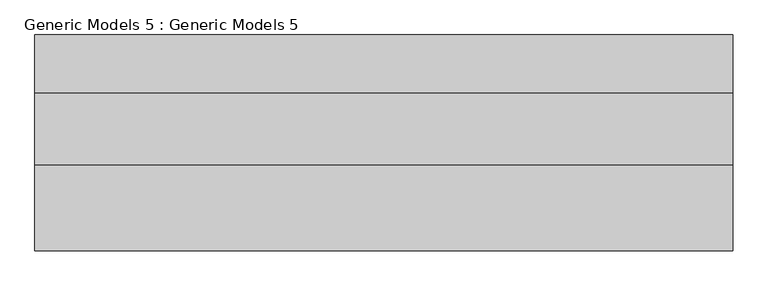
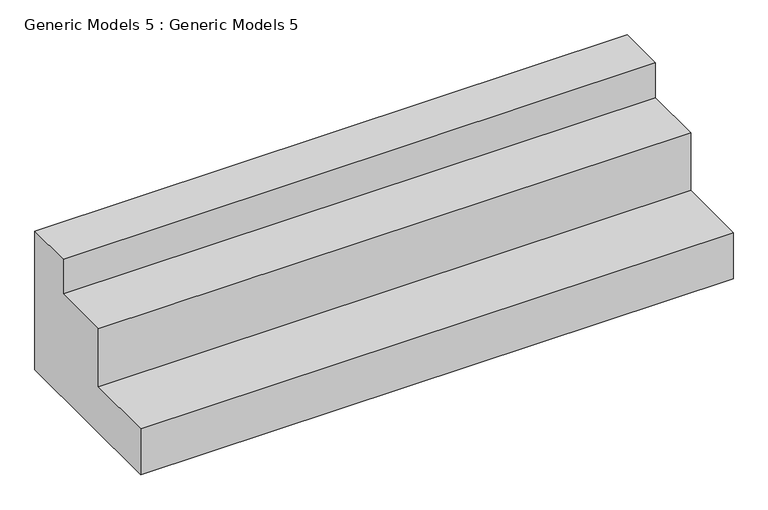
"""IFC4 building model written with IfcOpenShell, lengths in millimetres: proxy geometry, Generic Models 5 : Generic Models 5."""

from ifc_helpers import new_model, si_unit, frame, origin, place, context, project, spatial, polyline, outline, extrude, source, transform, mapped, element, save


def generic_models_5_generic_models_5_28bce95b(model_context):
    return source(origin(), model_context, "Body", "SweptSolid", [
        extrude(outline(polyline([(-4329.7340831, 0.0), (-4710.7340831, 0.0), (-4710.7340831, 101.6), (-4558.3340831, 101.6), (-4558.3340831, 228.6), (-4431.3340831, 228.6), (-4431.3340831, 304.8), (-4329.7340831, 304.8), (-4329.7340831, 0.0)])), frame((-8473.3860997, 0.0, 0.0), z_axis=(1.0, 0.0, 0.0), x_axis=(0.0, 1.0, 0.0)), (0.0, 0.0, 1.0), 1231.2238459),
    ])


if __name__ == "__main__":
    model = new_model("IFC4")
    model_context = context("Model", 3, world=origin())
    ifc_project = project(units=[si_unit("LENGTHUNIT", "METRE", prefix="MILLI")], contexts=[model_context])
    site = spatial("IfcSite", under=ifc_project)
    building = spatial("IfcBuilding", under=site)
    placement = place(None, origin())
    generic_models_5_generic_models_5_shape = generic_models_5_generic_models_5_28bce95b(model_context)
    element("IfcBuildingElementProxy", 1, Name="Generic Models 5 : Generic Models 5", ObjectType="Generic Models 5 : Generic Models 5", at=placement, inside=building, context=model_context, shape_type="MappedRepresentation", body=[
        mapped(generic_models_5_generic_models_5_shape, transform((0.0, 0.0, 0.0), x_axis=(1.0, 0.0, 0.0), y_axis=(0.0, 1.0, 0.0), z_axis=(0.0, 0.0, 1.0))),
    ])
    save(model, "model.ifc")
